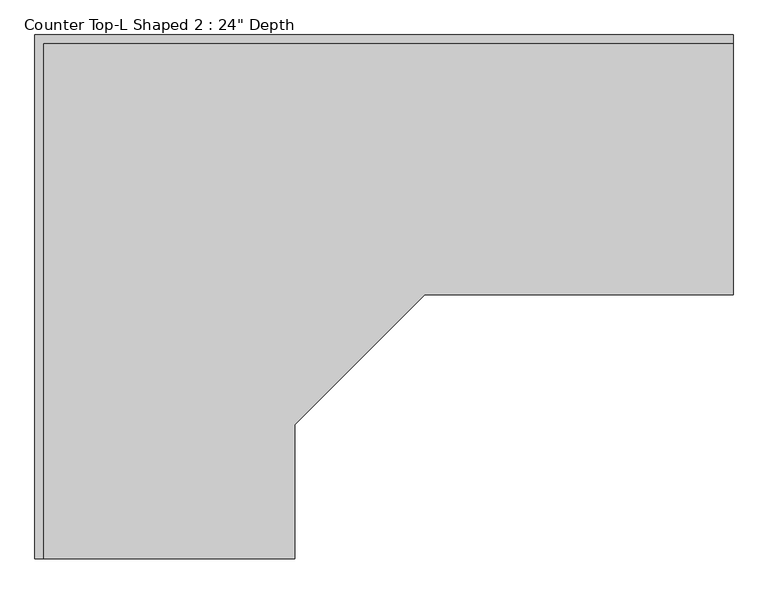
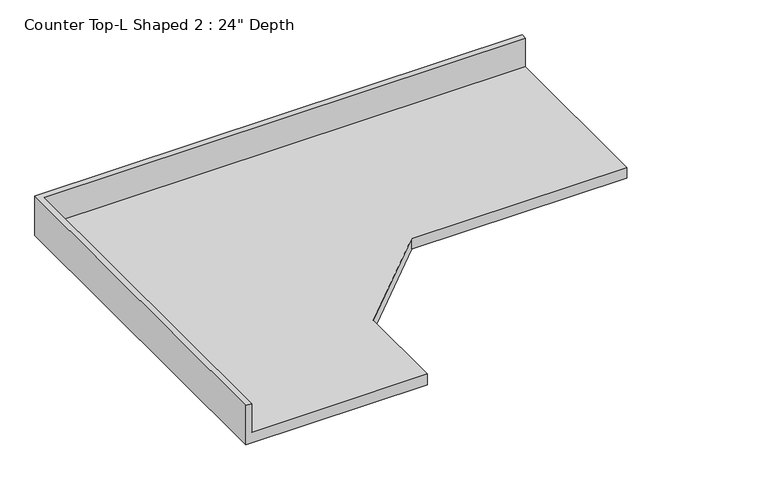
"""IFC4 building model written with IfcOpenShell, lengths in millimetres: furniture geometry."""

from ifc_helpers import new_model, si_unit, origin, place, context, project, spatial, faceted_brep, source, transform, mapped, element, save


def furniture_36cde3d8(model_context):
    return source(origin(), model_context, "Body", "Brep", [
        faceted_brep([(-590.8622951, -1228.8071879, 609.6), (-590.8622951, -914.4, 609.6), (-286.0622951, -609.6, 609.6), (437.1010039, -609.6, 609.6), (437.1010039, -19.05, 609.6), (-1181.4122951, -19.05, 609.6), (-1181.4122951, -1228.8071879, 609.6), (437.1010039, 0.0, 571.5), (437.1010039, -609.6, 571.5), (-286.0622951, -609.6, 571.5), (-590.8622951, -914.4, 571.5), (-590.8622951, -1228.8071879, 571.5), (-1200.4622951, -1228.8071879, 571.5), (-1200.4622951, 0.0, 571.5), (-1200.4622951, 0.0, 711.2), (437.1010039, 0.0, 711.2), (-1200.4622951, -1228.8071879, 711.2), (-1181.4122951, -1228.8071879, 711.2), (437.1010039, -19.05, 711.2), (-1181.4122951, -19.05, 711.2)], [[[0, 1, 2, 3, 4, 5, 6]], [[7, 8, 9, 10, 11, 12, 13]], [[7, 13, 14, 15]], [[13, 12, 16, 14]], [[16, 12, 11, 0, 6, 17]], [[1, 0, 11, 10]], [[2, 1, 10, 9]], [[3, 2, 9, 8]], [[8, 7, 15, 18, 4, 3]], [[14, 16, 17, 19, 18, 15]], [[4, 18, 19, 5]], [[19, 17, 6, 5]]]),
    ])


if __name__ == "__main__":
    model = new_model("IFC4")
    model_context = context("Model", 3, world=origin())
    ifc_project = project(units=[si_unit("LENGTHUNIT", "METRE", prefix="MILLI")], contexts=[model_context])
    site = spatial("IfcSite", under=ifc_project)
    building = spatial("IfcBuilding", under=site)
    placement = place(None, origin())
    furniture_shape = furniture_36cde3d8(model_context)
    element("IfcFurniture", 1, ObjectType="Counter Top-L Shaped 2 : 24\" Depth", at=placement, inside=building, context=model_context, shape_type="MappedRepresentation", body=[
        mapped(furniture_shape, transform((0.0, 0.0, 0.0), x_axis=(1.0, 0.0, 0.0), y_axis=(0.0, 1.0, 0.0), z_axis=(0.0, 0.0, 1.0))),
    ])
    save(model, "model.ifc")

# Revit data of these elements
# Type "Counter Top-L Shaped 2 : 24\" Depth"
#   Assembly Code = "C1030400"
#   Counter Thickness = 0' - 1 1/2"
#   Depth = 2' - 0"
#   Height = 2' - 0"
#   Length - Leg 1 [instance default] = 8' - 0"
#   Length - Leg 2 [instance default] = 6' - 0"
#   Counter Top Material = none
#   Default Elevation = 0
# Element 1 (IfcFurniture, "Counter Top-L Shaped 2 : 24\" Depth")
#   Length - Leg 1 = 5' - 4.471"
#   Length - Leg 2 = 4' - 0.37824"
#   Materials on its faces: "Counter Top"
# Materials
#   "Counter Top": class "Wood", colour RGB 226 177 128, transparency 0
